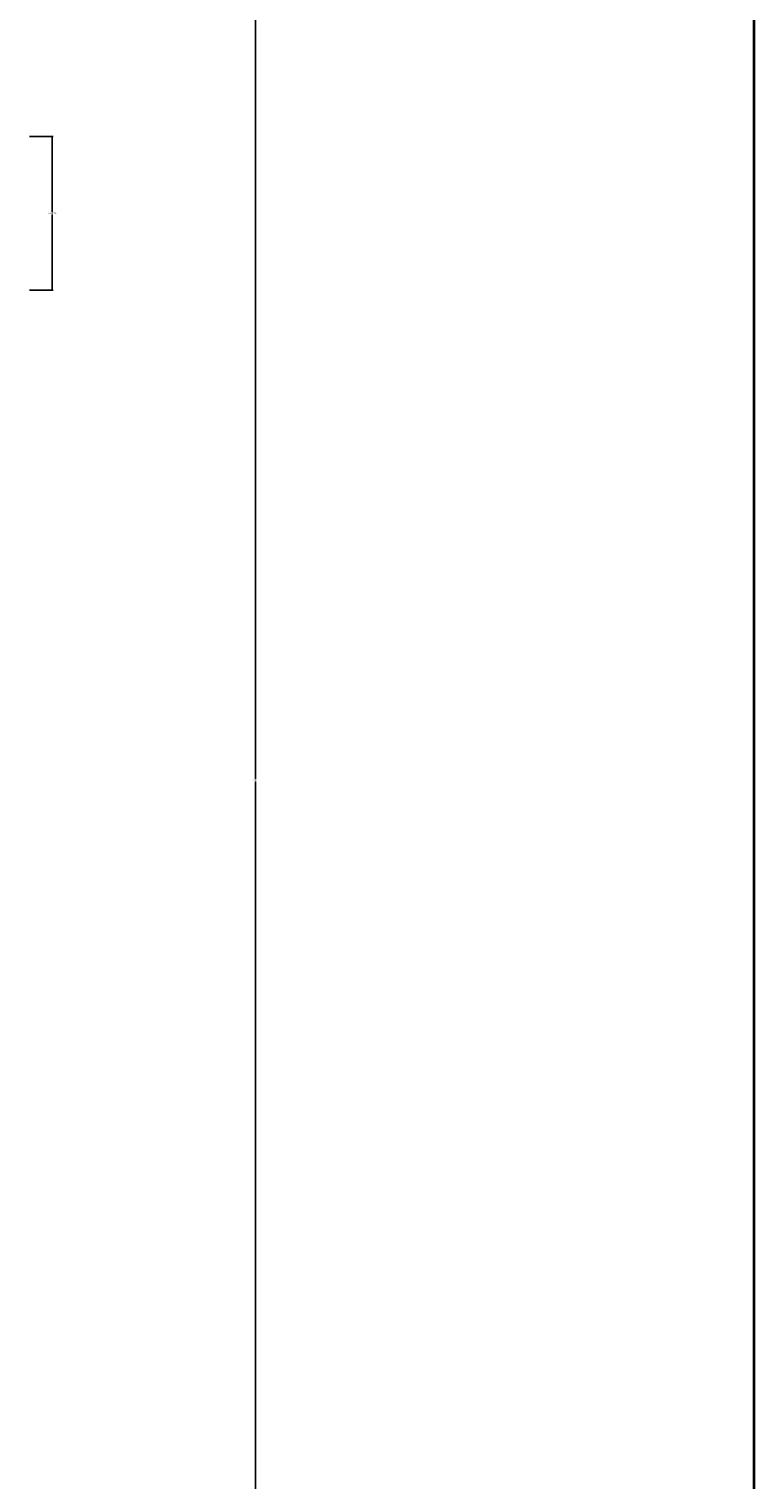
# Model space of a CAD drawing. Units: inches. Extents: x 2234 to 3001, y 1541 to 2386.
# Tile 11 of 12: x 2888 to 3001, y 1891 to 2118. Entities that reach past the tile are written whole.
import ezdxf

# ---------------------------------------------------------------- set-up
doc = ezdxf.new("R2010")
doc.units = ezdxf.units.IN
doc.layers.add('A-ANNO-DIMS', color=2, linetype='Continuous', lineweight=18)
doc.layers.add('A-ANNO-TTLB', color=7, linetype='Continuous', lineweight=35)
doc.styles.get("Standard").update_dxf_attribs({"font": 'arial.ttf'})
doc.dimstyles.get("Standard").update_dxf_attribs({"dimtxt": 0.18, "dimasz": 0.18, "dimexe": 0.18, "dimexo": 0.0625, "dimgap": 0.09, "dimtad": 0, "dimtih": 1, "dimtoh": 1, "dimdec": 4, "dimzin": 0, "dimdsep": 46, "dimtxsty": 'Standard', "dimcen": 0.09, "dimadec": 0, "dimazin": 0, "dimtfac": 1, "dimtdec": 4, "dimtofl": 0, "dimtmove": 0, "dimatfit": 3, "dimfxl": 1, "dimtolj": 1, "dimtzin": 0, "dimarcsym": 0})

# ---------------------------------------------------------------- blocks, each defined once
blk = doc.blocks.new('*D29')
at = {"layer": 'A-ANNO-DIMS', "color": 0, "lineweight": -2, "transparency": 16777216}
for p, q in [((2888.32, 2100.78), (2892.03, 2100.78)), ((2891.85, 2100.6), (2891.85, 2088.96)), ((2891.85, 2076.96), (2891.85, 2088.6)), ((2888.32, 2076.78), (2892.03, 2076.78))]:
    blk.add_line(p, q, dxfattribs=at)
at = {"layer": 'A-ANNO-DIMS', "color": 0, "transparency": 16777216}
for points in [[(2891.82, 2100.6), (2891.88, 2100.6), (2891.85, 2100.78)], [(2891.82, 2076.96), (2891.88, 2076.96), (2891.85, 2076.78)]]:
    blk.add_solid(points, dxfattribs=at)
at = {"layer": 'Defpoints', "color": 0, "transparency": 16777216}
for p in [(2888.25, 2100.78), (2888.25, 2076.78), (2891.85, 2076.78)]:
    blk.add_point(p, dxfattribs=at)
at = {"layer": 'A-ANNO-DIMS', "color": 0, "transparency": 16777216, "insert": (2891.85, 2088.78), "char_height": 0.18, "attachment_point": 5}
blk.add_mtext('\\A1;W-A 24 TYP.', dxfattribs=at)
blk = doc.blocks.new('*D62')
at = {"layer": 'A-ANNO-DIMS', "color": 0, "lineweight": -2, "transparency": 16777216}
for p, q in [((2888.32, 2298.61), (2923.78, 2298.61)), ((2923.6, 2298.43), (2923.6, 2000.54)), ((2923.6, 1702.29), (2923.6, 2000.18)), ((2888.32, 1702.11), (2923.78, 1702.11))]:
    blk.add_line(p, q, dxfattribs=at)
at = {"layer": 'A-ANNO-DIMS', "color": 0, "transparency": 16777216}
for points in [[(2923.57, 2298.43), (2923.63, 2298.43), (2923.6, 2298.61)], [(2923.57, 1702.29), (2923.63, 1702.29), (2923.6, 1702.11)]]:
    blk.add_solid(points, dxfattribs=at)
at = {"layer": 'Defpoints', "color": 0, "transparency": 16777216}
for p in [(2888.25, 2298.61), (2923.6, 2298.61), (2888.25, 1702.11)]:
    blk.add_point(p, dxfattribs=at)
at = {"layer": 'A-ANNO-DIMS', "color": 0, "transparency": 16777216, "insert": (2923.6, 2000.36), "char_height": 0.18, "attachment_point": 5}
blk.add_mtext('\\A1;596.5', dxfattribs=at)

msp = doc.modelspace()

# ---------------------------------------------------------------- linework, layer by layer
at = {"layer": 'A-ANNO-TTLB'}
msp.add_lwpolyline([(2233.5367, 2385.7012), (3001.3383, 2385.7012), (3001.3383, 1541.435), (2233.5367, 1541.435)], close=True, dxfattribs=at)

# ---------------------------------------------------------------- dimensions: what is measured, and where the dimension line sits
at = {"layer": 'A-ANNO-DIMS'}
dim = msp.add_linear_dim(base=(2923.6034, 2298.611), p1=(2888.2534, 1702.111), p2=(2888.2534, 2298.611), angle=90, dimstyle='Standard', override={"dimdec": 1, "dimlfac": 1, "dimrnd": 0, "dimzin": 0, "dimdsep": 46, "dimlunit": 2}, dxfattribs=at)
dim.commit()
dim.dimension.update_dxf_attribs({"geometry": '*D62', "text_midpoint": (2923.6034, 2000.361)})
dim = msp.add_linear_dim(base=(2891.8534, 2076.7794), p1=(2888.2534, 2100.7794), p2=(2888.2534, 2076.7794), angle=270, text='W-A <> TYP.', dimstyle='Standard', override={"dimdec": 0, "dimlfac": 1, "dimrnd": 0, "dimzin": 0, "dimdsep": 46, "dimlunit": 2}, dxfattribs=at)
dim.commit()
dim.dimension.update_dxf_attribs({"geometry": '*D29', "text_midpoint": (2891.8534, 2088.7794)})

doc.saveas('drawing.dxf')
